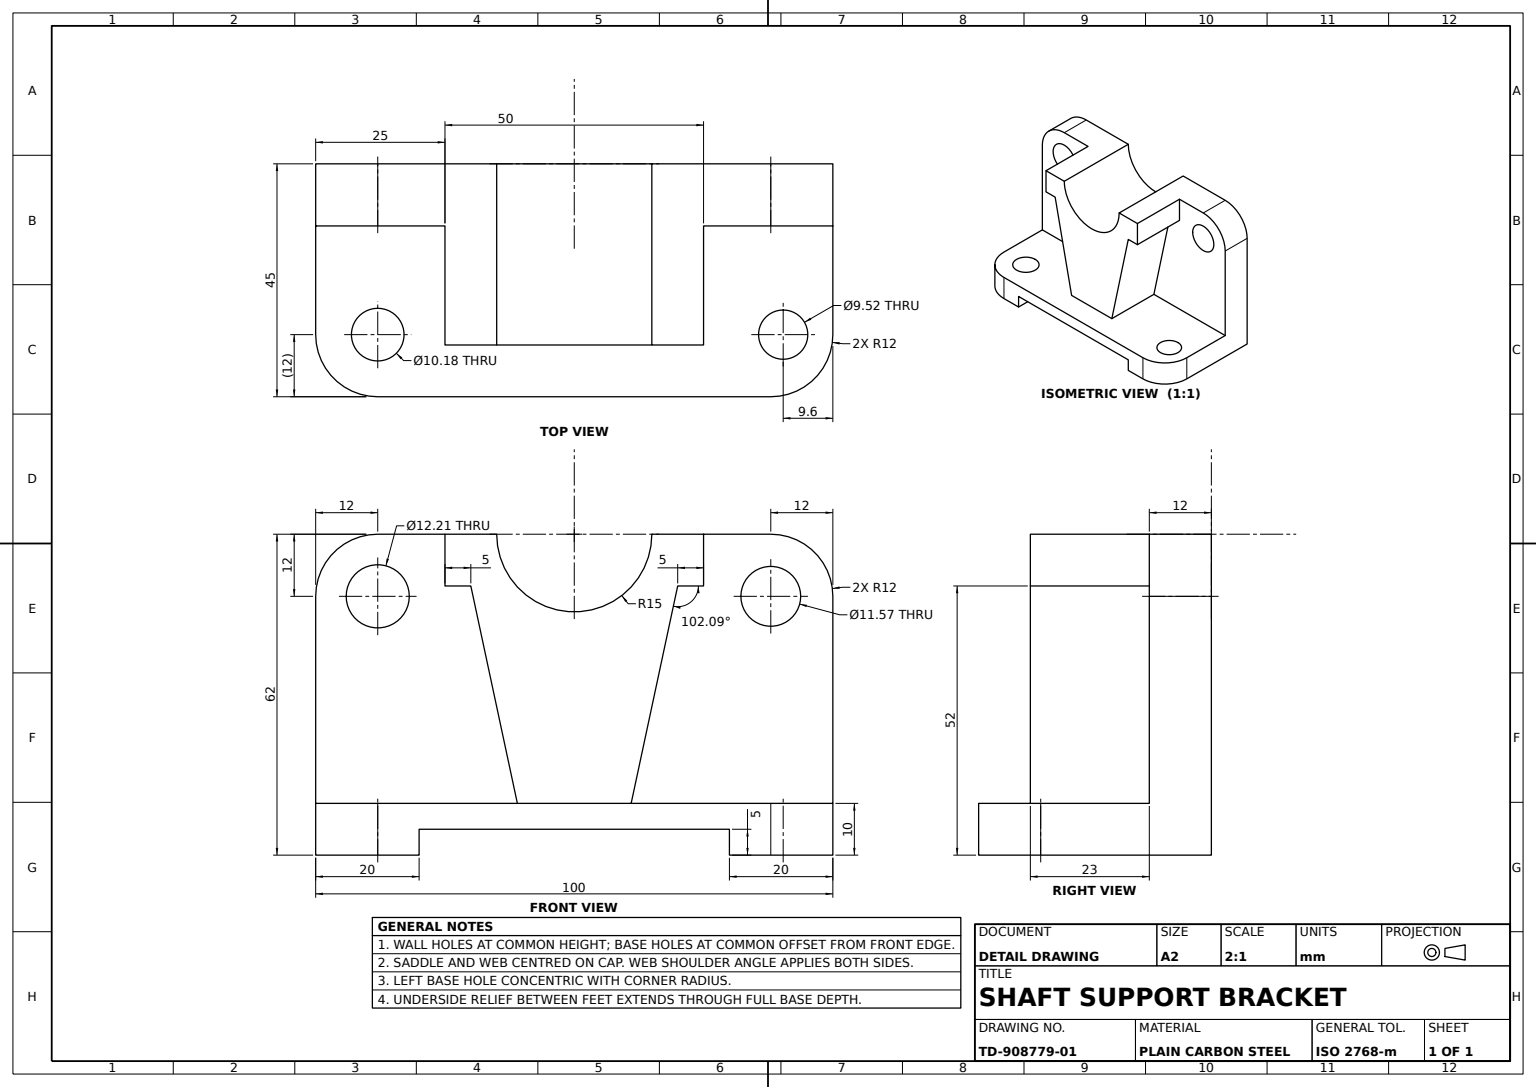
from build123d import *

# Parameters (mm, degrees)
BASE_PLATE_DEPTH               = 22.5
BACK_WALL_SKETCH_W             = 12
BACK_WALL_SKETCH_H             = 52
BACK_WALL_DEPTH                = 100
SADDLE_SUPPORT_DEPTH           = 23
WALL_HOLES_SKETCH_R            = 15
WALL_HOLES_SKETCH_R_2          = 6.102513624
WALL_HOLES_SKETCH_R_3          = 5.783086219
WALL_HOLES_DEPTH               = 123.200654663
WALL_CORNER_FILLETS_R12_R      = 12
BASE_MOUNTING_HOLES_SKETCH_R   = 5.090614353
BASE_MOUNTING_HOLES_SKETCH_R_2 = 4.76218762
BASE_MOUNTING_HOLES_DEPTH      = 115.935851674


with BuildPart() as part:
    # Base Plate Profile → Base Plate (new, symmetric)
    with BuildSketch(Plane.XY):
        Polygon((0, 0), (20, 0), (20, 5), (80, 5), (80, 0), (100, 0), (100, 10), (0, 10), align=None)
    extrude(amount=BASE_PLATE_DEPTH, both=True)

    # Back Wall Sketch → Back Wall (add)
    with BuildSketch(Plane(origin=(100, 0, 0), x_dir=(0, 0, -1), z_dir=(1, 0, 0))):
        with Locations((16.5, 36)):
            Rectangle(BACK_WALL_SKETCH_W, BACK_WALL_SKETCH_H)
    extrude(amount=-BACK_WALL_DEPTH)

    # Saddle Support Profile → Saddle Support (add)
    with BuildSketch(Plane.XY.offset(-10.5)):
        with BuildLine():
            Line((39, 10), (61, 10))
            Line((61, 10), (70, 52))
            Line((70, 52), (75, 52))
            Line((75, 52), (75, 62))
            Line((75, 62), (65, 62))
            ThreePointArc((65, 62), (50, 47), (35, 62))
            Line((35, 62), (25, 62))
            Line((25, 62), (25, 52))
            Line((25, 52), (30, 52))
            Line((30, 52), (39, 10))
        make_face()
    extrude(amount=SADDLE_SUPPORT_DEPTH)

    # Wall Holes Sketch → Wall Holes (cut, through all)
    with BuildSketch(Plane.XY.offset(-10.5)):
        with Locations((50, 62)):
            Circle(WALL_HOLES_SKETCH_R)
        with Locations((12, 50)):
            Circle(WALL_HOLES_SKETCH_R_2)
        with Locations((88, 50)):
            Circle(WALL_HOLES_SKETCH_R_3)
    extrude(amount=-WALL_HOLES_DEPTH, mode=Mode.SUBTRACT)

    # Wall Corner Fillets R12
    wall_corner_fillets_r12_edges = [part.edges().sort_by_distance(p)[0] for p in [
        (0, 5, 22.5),
        (100, 62, -16.5),
        (0, 62, -16.5),
        (100, 5, 22.5),
    ]]
    fillet(wall_corner_fillets_r12_edges, radius=WALL_CORNER_FILLETS_R12_R)

    # Base Mounting Holes Sketch → Base Mounting Holes (cut, through all)
    with BuildSketch(Plane(origin=(0, 10, 0), x_dir=(1, 0, 0), z_dir=(0, 1, 0))):
        with Locations(Location((12, -10.5, 0), (0, 0, 270))):
            Circle(BASE_MOUNTING_HOLES_SKETCH_R)
        with Locations(Location((90.396488088, -10.5, 0), (0, 0, 270))):
            Circle(BASE_MOUNTING_HOLES_SKETCH_R_2)
    extrude(amount=-BASE_MOUNTING_HOLES_DEPTH, mode=Mode.SUBTRACT)


solid = part.part
